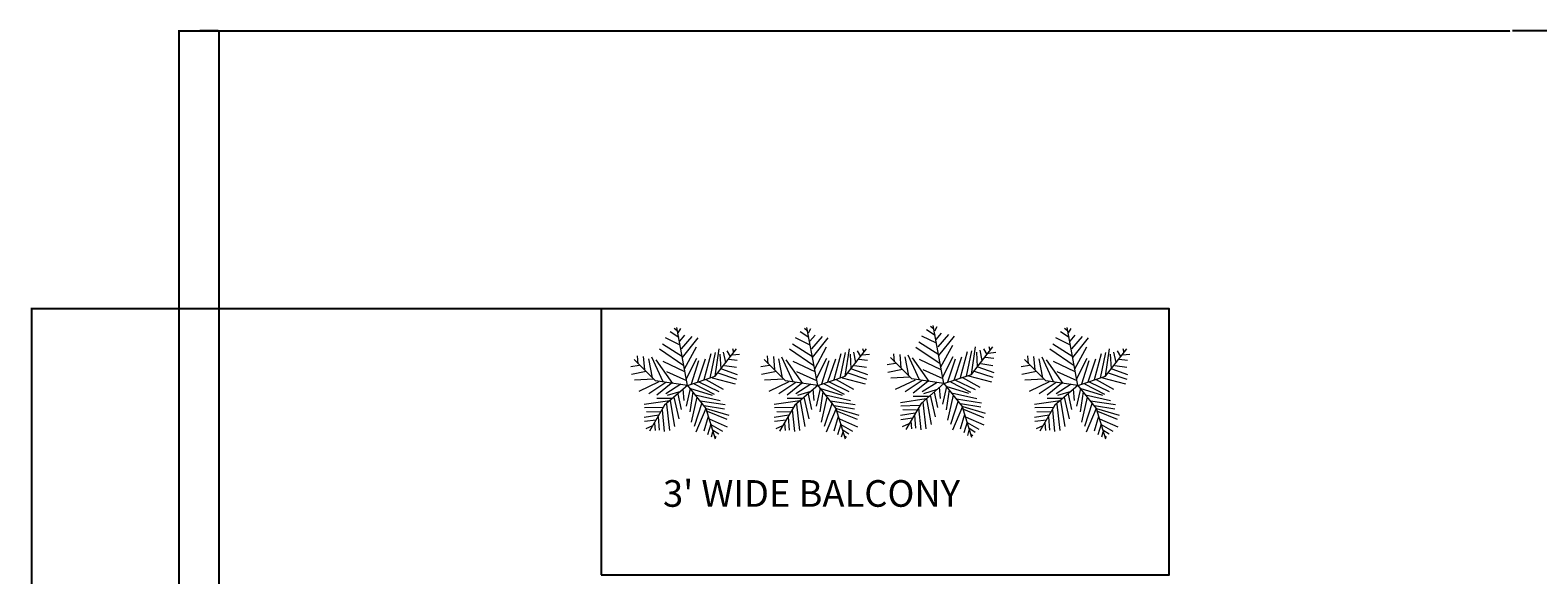
# Model space of a CAD drawing. Units: inches. Extents: x 4159 to 4826, y 299 to 1026.
# Tile 36 of 37: x 4159 to 4498, y 903 to 1026. Entities that reach past the tile are written whole.
import ezdxf

# ---------------------------------------------------------------- set-up
doc = ezdxf.new("R2010")
doc.units = ezdxf.units.IN
for name, color, linetype, lineweight in [('A-ANNO-DIMS', 2, 'Continuous', 18), ('A-AREA-IDEN', 7, 'Continuous', 18), ('A-FLOR-BALC', 7, 'Continuous', 25), ('L-PLNT', 94, 'Continuous', 13)]:
    doc.layers.add(name, color=color, linetype=linetype, lineweight=lineweight)
doc.styles.get("Standard").update_dxf_attribs({"font": 'arial.ttf'})
doc.dimstyles.get("Standard").update_dxf_attribs({"dimtxt": 0.18, "dimasz": 0.18, "dimexe": 0.18, "dimexo": 0.0625, "dimgap": 0.09, "dimtad": 0, "dimtih": 1, "dimtoh": 1, "dimdec": 4, "dimzin": 0, "dimdsep": 46, "dimtxsty": 'Standard', "dimcen": 0.09, "dimadec": 0, "dimazin": 0, "dimtfac": 1, "dimtdec": 4, "dimtofl": 0, "dimtmove": 0, "dimatfit": 3, "dimfxl": 1, "dimtolj": 1, "dimtzin": 0, "dimarcsym": 0})

# ---------------------------------------------------------------- blocks, each defined once
blk = doc.blocks.new('*U12')
for p, q in [((-7.288, 39.707), (-21.778, 46.673)), ((-8.737, 47.138), (-17.069, 52.711)), ((-10.186, 53.64), (-13.084, 55.962)), ((0, 0), (-10.5, 57)), ((-9.099, 51.782), (-6.563, 55.962)), ((-7.65, 43.423), (-2.578, 49.46)), ((-5.839, 35.992), (4.667, 48.067)), ((-5.114, 27.632), (10.463, 46.673)), ((-3.665, 19.273), (-27.574, 35.527)), ((-5.114, 28.097), (-24.676, 40.636)), ((-2.941, 16.486), (8.652, 37.85)), ((16.259, 5.805), (23.142, 31.348)), ((22.055, 7.198), (27.489, 32.277)), ((27, 9), (48, 36)), ((27.127, 9.056), (31.112, 35.992)), ((31.836, 30.883), (32.561, 16.486)), ((35.096, 32.741), (37.27, 22.524)), ((38.719, 34.134), (41.979, 28.561)), ((43.791, 29.954), (51.036, 30.883)), ((44.153, 36.456), (45.239, 32.741)), ((-47.498, 19.737), (-55.83, 18.344)), ((-31.5, 4.5), (-52.5, 25.5)), ((-48.585, 21.131), (-49.309, 29.026)), ((-43.513, 28.561), (-42.427, 15.558)), ((-38.442, 26.239), (-34.819, 7.663)), ((-35.544, 28.097), (-24.314, 3.947)), ((-14.533, 2.09), (-30.834, 25.31)), ((-24.314, 23.917), (-2.941, 13.7)), ((-1.129, 6.734), (9.014, 26.704)), ((3.942, 1.625), (11.187, 24.381)), ((10.101, 3.483), (17.708, 26.239)), ((33.285, 16.486), (48.862, 10.913)), ((36.183, 19.737), (48.137, 17.88)), ((40.53, 25.775), (48.862, 24.846)), ((-40.615, 13.7), (-55.105, 10.913)), ((-33.37, 6.269), (-52.207, 5.34)), ((-28.299, 3.483), (-47.86, -5.805)), ((-21.416, 3.018), (-38.079, -8.128)), ((0, 0), (-31.5, 4.5)), ((-15.982, 2.09), (-30.11, -9.521)), ((0, 0), (-22.5, -19.5)), ((-6.563, 1.161), (-21.416, -8.128)), ((-20.691, 13.7), (-1.129, 4.876)), ((0, 0), (27, 9)), ((0, 0), (18, -22.5)), ((6.478, 1.625), (26.04, -8.592)), ((11.187, 3.483), (30.749, -5.805)), ((18.07, 5.805), (35.096, -3.483)), ((24.229, 7.663), (46.688, 1.625)), ((29.662, 12.307), (48.137, 6.269)), ((-15.257, -12.772), (-30.11, -12.772)), ((-6.563, -5.805), (-19.967, -9.985)), ((-13.446, -11.378), (-8.737, -32.741)), ((-9.461, -8.592), (-6.201, -23.453)), ((-4.752, -3.483), (-3.665, -14.629)), ((2.493, -3.019), (-1.491, -20.202)), ((1.769, -2.555), (24.229, -9.521)), ((5.029, -6.27), (2.131, -25.775)), ((9.014, -11.378), (3.58, -35.992)), ((7.565, -9.056), (32.198, -14.629)), ((-17.431, -15.094), (-42.789, -18.809)), ((-28.299, -29.026), (-42.789, -31.348)), ((-24.314, -21.596), (-42.427, -22.06)), ((-26.849, -26.24), (-40.253, -25.775)), ((-22.5, -19.5), (-37.5, -45)), ((-25.038, -23.918), (-22.865, -45.281)), ((-20.691, -18.345), (-17.793, -44.352)), ((-17.069, -15.094), (-12.721, -40.172)), ((14.085, -16.951), (6.478, -40.172)), ((18.07, -22.524), (8.289, -45.745)), ((12.274, -15.094), (36.907, -18.809)), ((16.259, -19.738), (36.183, -22.989)), ((18, -22.5), (27, -52.5)), ((18.433, -22.524), (40.53, -29.026)), ((19.157, -25.311), (38.719, -33.206)), ((-30.834, -34.135), (-42.427, -35.528)), ((-34.457, -39.708), (-40.978, -42.494)), ((-32.646, -36.921), (-31.921, -44.352)), ((-29.023, -30.884), (-27.936, -43.887)), ((20.244, -30.419), (15.897, -44.816)), ((22.78, -37.85), (19.519, -48.532)), ((21.331, -32.741), (39.081, -40.636)), ((22.78, -38.314), (34.372, -44.816)), ((24.591, -43.423), (30.749, -47.603)), ((24.591, -45.745), (23.142, -50.854)), ((26.764, -49.925), (28.213, -50.854))]:
    blk.add_line(p, q)
blk = doc.blocks.new('*D43')
at = {"layer": 'A-ANNO-DIMS', "color": 0, "lineweight": -2, "transparency": 16777216}
for p, q in [((4192.31, 903.32), (4192.31, 1025.84)), ((4192.49, 1025.66), (4492.02, 1025.66)), ((4792.13, 1025.66), (4492.6, 1025.66)), ((4792.31, 903.32), (4792.31, 1025.84))]:
    blk.add_line(p, q, dxfattribs=at)
at = {"layer": 'A-ANNO-DIMS', "color": 0, "transparency": 16777216}
for points in [[(4192.49, 1025.69), (4192.49, 1025.63), (4192.31, 1025.66)], [(4792.13, 1025.69), (4792.13, 1025.63), (4792.31, 1025.66)]]:
    blk.add_solid(points, dxfattribs=at)
at = {"layer": 'Defpoints', "color": 0, "transparency": 16777216}
for p in [(4792.31, 1025.66), (4192.31, 903.25), (4792.31, 903.25)]:
    blk.add_point(p, dxfattribs=at)
at = {"layer": 'A-ANNO-DIMS', "color": 0, "transparency": 16777216, "insert": (4492.31, 1025.66), "char_height": 0.18, "attachment_point": 5}
blk.add_mtext('\\A1;600', dxfattribs=at)
blk = doc.blocks.new('*D44')
at = {"layer": 'A-ANNO-DIMS', "color": 0, "lineweight": -2, "transparency": 16777216}
for p, q in [((4287.26, 963.09), (4158.88, 963.09)), ((4159.06, 962.91), (4159.06, 647.83)), ((4159.06, 332.38), (4159.06, 647.46)), ((4447.25, 332.2), (4158.88, 332.2))]:
    blk.add_line(p, q, dxfattribs=at)
at = {"layer": 'A-ANNO-DIMS', "color": 0, "transparency": 16777216}
for points in [[(4159.03, 962.91), (4159.09, 962.91), (4159.06, 963.09)], [(4159.03, 332.38), (4159.09, 332.38), (4159.06, 332.2)]]:
    blk.add_solid(points, dxfattribs=at)
at = {"layer": 'Defpoints', "color": 0, "transparency": 16777216}
for p in [(4287.33, 963.09), (4159.06, 332.2), (4447.31, 332.2)]:
    blk.add_point(p, dxfattribs=at)
at = {"layer": 'A-ANNO-DIMS', "color": 0, "transparency": 16777216, "insert": (4159.06, 647.64), "char_height": 0.18, "attachment_point": 5}
blk.add_mtext('\\A1;630.9', dxfattribs=at)
blk = doc.blocks.new('*D50')
at = {"layer": 'A-ANNO-DIMS', "color": 0, "lineweight": -2, "transparency": 16777216}
for p, q in [((4192.31, 392.32), (4192.31, 1025.84)), ((4192.49, 1025.66), (4196.66, 1025.66)), ((4201.13, 1025.66), (4196.96, 1025.66)), ((4201.31, 401.32), (4201.31, 1025.84))]:
    blk.add_line(p, q, dxfattribs=at)
at = {"layer": 'A-ANNO-DIMS', "color": 0, "transparency": 16777216}
for points in [[(4192.49, 1025.69), (4192.49, 1025.63), (4192.31, 1025.66)], [(4201.13, 1025.69), (4201.13, 1025.63), (4201.31, 1025.66)]]:
    blk.add_solid(points, dxfattribs=at)
at = {"layer": 'Defpoints', "color": 0, "transparency": 16777216}
for p in [(4201.31, 1025.66), (4201.31, 401.25), (4192.31, 392.25)]:
    blk.add_point(p, dxfattribs=at)
at = {"layer": 'A-ANNO-DIMS', "color": 0, "transparency": 16777216, "insert": (4196.81, 1025.66), "char_height": 0.18, "attachment_point": 5}
blk.add_mtext('\\A1;9', dxfattribs=at)

msp = doc.modelspace()

# ---------------------------------------------------------------- linework, layer by layer
at = {"layer": 'A-FLOR-BALC'}
msp.add_lwpolyline([(4287.326, 903.254), (4415.251, 903.254), (4415.251, 963.093), (4287.326, 963.093)], close=True, dxfattribs=at)

# ---------------------------------------------------------------- block references
at = {"layer": 'L-PLNT', "xscale": 0.2292012274639507, "yscale": 0.2292012274639507, "zscale": 0.2292012274639507}
for p in [(4306.812, 945.873), (4336.116, 945.873), (4364.557, 946.304), (4394.722, 945.873)]:
    msp.add_blockref('*U12', p, dxfattribs=at)

# ---------------------------------------------------------------- texts
at = {"layer": 'A-AREA-IDEN'}
msp.add_text("3' WIDE BALCONY", height=6, dxfattribs=at).set_placement((4301.282, 918.57))

# ---------------------------------------------------------------- dimensions: what is measured, and where the dimension line sits
at = {"layer": 'A-ANNO-DIMS'}
for base, p1, p2, picture, middle in [((4792.31, 1025.662), (4192.31, 903.254), (4792.31, 903.254), '*D43', (4492.31, 1025.662)), ((4201.31, 1025.662), (4192.31, 392.254), (4201.31, 401.254), '*D50', (4196.81, 1025.662))]:
    dim = msp.add_linear_dim(base=base, p1=p1, p2=p2, dimstyle='Standard', override={"dimdec": 0, "dimlfac": 1, "dimrnd": 0, "dimzin": 0, "dimdsep": 46, "dimlunit": 2}, dxfattribs=at)
    dim.commit()
    dim.dimension.update_dxf_attribs({"geometry": picture, "text_midpoint": middle})
dim = msp.add_linear_dim(base=(4159.06, 332.195), p1=(4287.326, 963.093), p2=(4447.31, 332.195), angle=90, dimstyle='Standard', override={"dimdec": 1, "dimlfac": 1, "dimrnd": 0, "dimzin": 0, "dimdsep": 46, "dimlunit": 2}, dxfattribs=at)
dim.commit()
dim.dimension.update_dxf_attribs({"geometry": '*D44', "text_midpoint": (4159.06, 647.644)})

doc.saveas('drawing.dxf')
